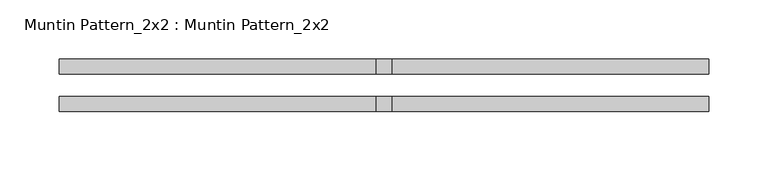
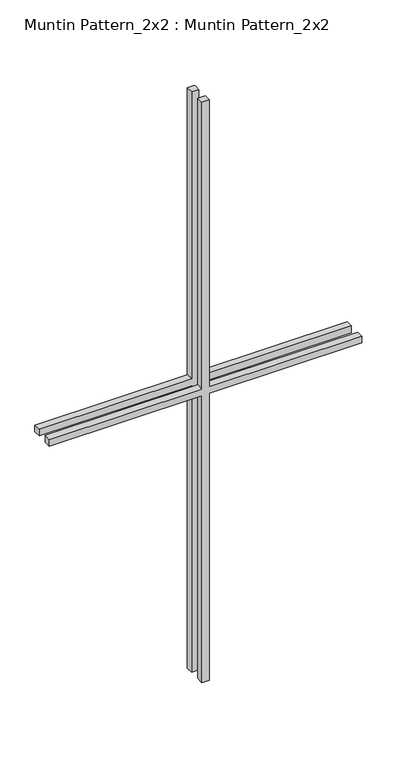
"""IFC4 building model written with IfcOpenShell, lengths in millimetres: proxy geometry, Muntin Pattern_2x2 : Muntin Pattern_2x2."""

from ifc_helpers import new_model, si_unit, frame, origin, place, context, project, spatial, polyline, outline, extrude, source, transform, mapped, element, save


def muntin_pattern_2x2_muntin_pattern_2x2_811e8f4b(model_context):
    return source(origin(), model_context, "Body", "SweptSolid", [
        extrude(outline(polyline([(546.1, -6.35), (546.1, -274.6375), (533.4, -274.6375), (533.4, -6.35), (0.0, -6.35), (0.0, 6.35), (533.4, 6.35), (533.4, 274.6375), (546.1, 274.6375), (546.1, 6.35), (1079.5, 6.35), (1079.5, -6.35), (546.1, -6.35)])), frame((0.0, -22.225, 0.0), z_axis=(0.0, 1.0, 0.0), x_axis=(0.0, 0.0, 1.0)), (0.0, 0.0, 1.0), 12.7),
        extrude(outline(polyline([(546.1, -6.35), (546.1, -274.6375), (533.4, -274.6375), (533.4, -6.35), (0.0, -6.35), (0.0, 6.35), (533.4, 6.35), (533.4, 274.6375), (546.1, 274.6375), (546.1, 6.35), (1079.5, 6.35), (1079.5, -6.35), (546.1, -6.35)])), frame((0.0, 9.525, 0.0), z_axis=(0.0, 1.0, 0.0), x_axis=(0.0, 0.0, 1.0)), (0.0, 0.0, 1.0), 12.7),
    ])


if __name__ == "__main__":
    model = new_model("IFC4")
    model_context = context("Model", 3, world=origin())
    ifc_project = project(units=[si_unit("LENGTHUNIT", "METRE", prefix="MILLI")], contexts=[model_context])
    site = spatial("IfcSite", under=ifc_project)
    building = spatial("IfcBuilding", under=site)
    placement = place(None, origin())
    muntin_pattern_2x2_muntin_pattern_2x2_shape = muntin_pattern_2x2_muntin_pattern_2x2_811e8f4b(model_context)
    element("IfcBuildingElementProxy", 1, Name="Muntin Pattern_2x2 : Muntin Pattern_2x2", ObjectType="Muntin Pattern_2x2 : Muntin Pattern_2x2", at=placement, inside=building, context=model_context, shape_type="MappedRepresentation", body=[
        mapped(muntin_pattern_2x2_muntin_pattern_2x2_shape, transform((0.0, 0.0, 0.0), x_axis=(1.0, 0.0, 0.0), y_axis=(0.0, 1.0, 0.0), z_axis=(0.0, 0.0, 1.0))),
    ])
    save(model, "model.ifc")

# Revit data of these elements
# Type "Muntin Pattern_2x2 : Muntin Pattern_2x2"
#   Width [instance default] = 4' - 0"
#   Thickness = 0' - 0 1/2"
#   Height [instance default] = 4' - 0"
#   Distance = 0' - 0 3/4"
#   Interior Material [instance default] = none
#   Exterior Material [instance default] = none
#   Default Elevation = 0
# Element 1 (IfcBuildingElementProxy, "Muntin Pattern_2x2 : Muntin Pattern_2x2")
#   Width = 1' - 9 5/8"
#   Height = 3' - 6 1/2"
#   Interior Material = Wood - Stained
#   Exterior Material = Clad - White
#   Materials on its faces: "Clad - White", "Wood - Stained"
# Materials
#   "Clad - White": class "Wood", colour RGB 242 242 238, transparency 0, Cost = 0
#   "Wood - Stained": class "Wood", colour RGB 224 178 126, transparency 0, Cost = 0
